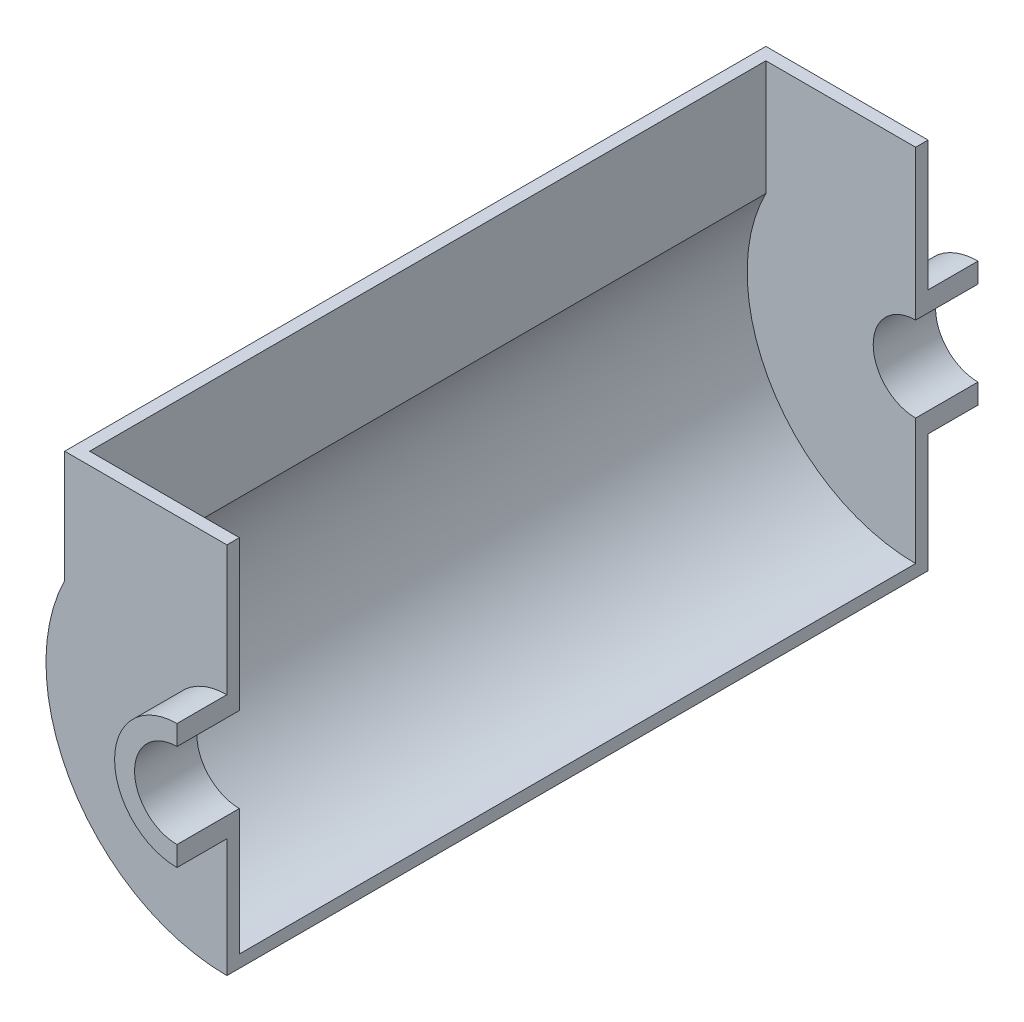
SolidWorks part; units mm, degrees
material "Plain Carbon Steel"
ref_plane "Front Plane" through (0, 0, 0) normal (0, 0, 1) x (1, 0, 0)
ref_plane "Top Plane" through (0, 0, 0) normal (0, 1, 0) x (1, 0, 0)
ref_plane "Right Plane" through (0, 0, 0) normal (1, 0, 0) x (0, 0, -1)
sketch "Trough Profile Sketch" plane through (0, 0, 0) normal (0, 0, 1) x (1, 0, 0)
  line L0 (0, 25) -> (0, -25)
  arc A0 (0, 25) -> (0, -25) centre (0, 0) ccw
  arc A1 (0, 17) -> (0, -17) centre (0, 0) ccw
  dimension "D1" = 50
  dimension "D2" = 34
extrude "Trough Shell" add sketch "Trough Profile Sketch" along normal blind 20 and the other way blind 5 contours A1 L0 A0
sketch "End Plate Sketch" plane through (0, 0, 0) normal (0, 0, 1) x (1, 0, 0)
  line L0 (0, 25) -> (0, 77)
  line L1 (0, 77) -> (-65, 77)
  line L2 (-65, 77) -> (-65, 32.1131)
  line L3 (0, -25) -> (0, -72.5)
  arc A0 (0, 25) -> (0, -25) centre (0, 0) ccw construction
  arc A1 (0, 25) -> (0, -25) centre (0, 0) ccw
  arc A2 (-65, 32.1131) -> (0, -72.5) centre (0, 0) ccw
  dimension "D3" = 72.5
  dimension "D1" = 52
  dimension "D2" = 65
extrude "End Plate" add sketch "End Plate Sketch" against normal blind 5
ref_plane "Plane1" through (0, 0, -140.5) normal (0, 0, 1) x (1, 0, 0)
mirror "End Plate Mirror" about plane through (0, 0, -140.5) normal (0, 0, 1) of bodies 102
sketch "Side Wall Sketch" plane through (0, 0, -5) normal (0, 0, -1) x (-1, 0, 0)
  line L0 (65, 77) -> (65, 32.1131) construction
  line L1 (65, 77) -> (65, 32.1131)
  line L2 (60, 77) -> (60, 30.9233)
  line L3 (65, 77) -> (60, 77)
  line L4 (0, -72.5) -> (0, -67.5)
  arc A0 (0, -72.5) -> (65, 32.1131) centre (0, 0) ccw construction
  arc A1 (0, -72.5) -> (65, 32.1131) centre (0, 0) ccw
  arc A2 (0, -67.5) -> (60, 30.9233) centre (0, 0) ccw
  dimension "D1" = 5
extrude "Side Walls" add sketch "Side Wall Sketch" along normal up to next
